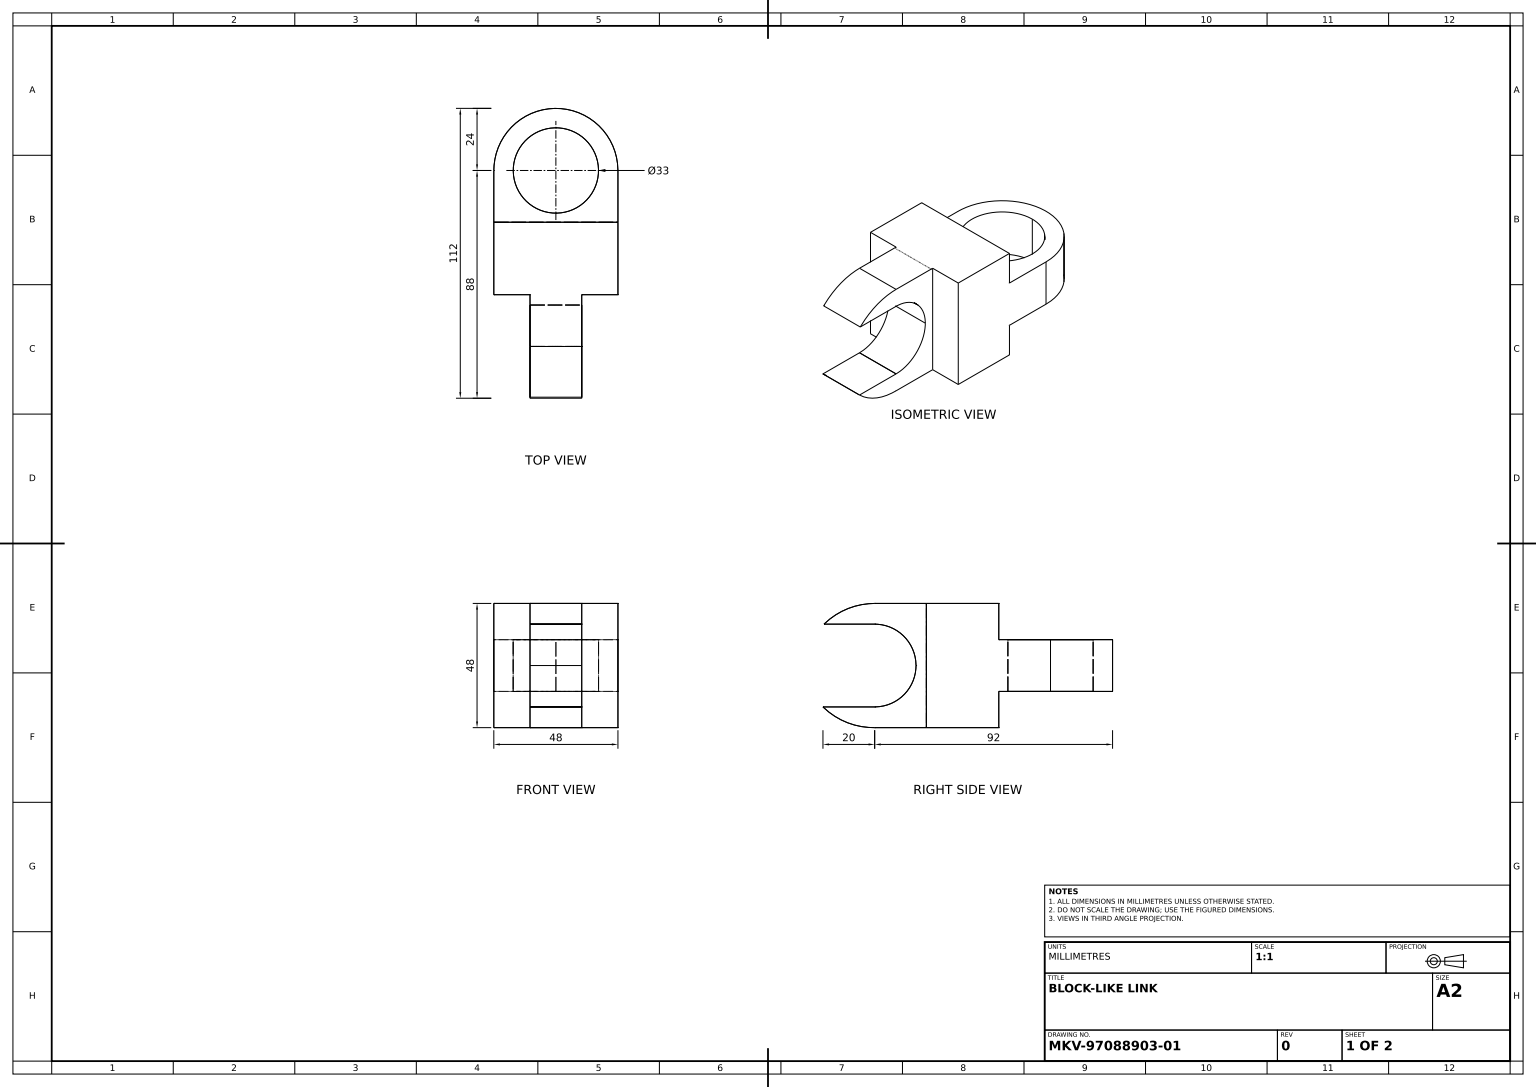
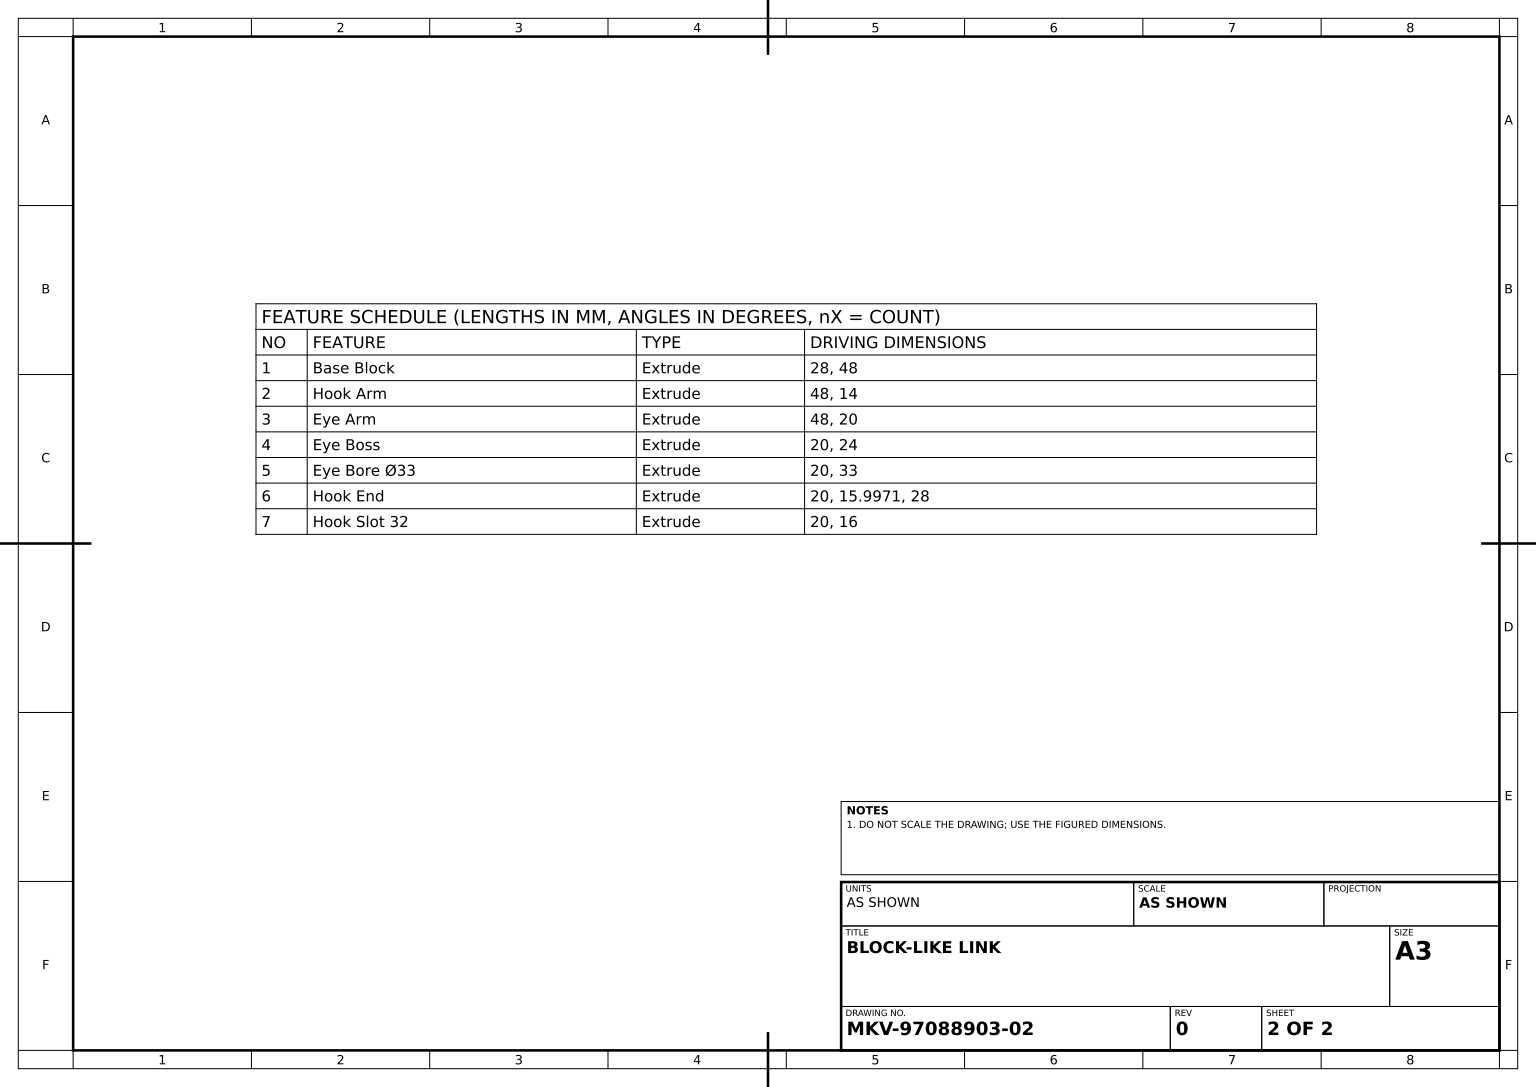
from build123d import *

# Parameters (mm, degrees)
BASE_BLOCK_SKETCH_W = 48
BASE_BLOCK_SKETCH_H = 48
BASE_BLOCK_DEPTH    = 28
HOOK_ARM_DEPTH      = 48
EYE_ARM_DEPTH       = 48
EYE_BOSS_DEPTH      = 20
EYE_BORE_SKETCH_R   = 16.5
EYE_BORE_33_DEPTH   = 20
HOOK_END_DEPTH      = 20
HOOK_SLOT_32_DEPTH  = 20


with BuildPart() as part:
    # Base Block Sketch → Base Block (new body)
    with BuildSketch(Plane.XY):
        with Locations((24, -24)):
            Rectangle(BASE_BLOCK_SKETCH_W, BASE_BLOCK_SKETCH_H)
    extrude(amount=BASE_BLOCK_DEPTH)

    # Hook Arm Sketch → Hook Arm (add)
    with BuildSketch(Plane(origin=(0, 0, 0), x_dir=(1, 0, 0), z_dir=(0, 1, 0))):
        Polygon((34, -28), (24, -28), (14, -28), (14, -48), (34, -48), align=None)
    extrude(amount=-HOOK_ARM_DEPTH)

    # Eye Arm Sketch → Eye Arm (add)
    with BuildSketch(Plane(origin=(48, 0, 0), x_dir=(0, 0, -1), z_dir=(1, 0, 0))):
        Polygon((0, -24), (0, -14), (20, -14), (20, -34), (0, -34), align=None)
    extrude(amount=-EYE_ARM_DEPTH)

    # Eye Boss Sketch → Eye Boss (add)
    with BuildSketch(Plane(origin=(0, -14, 0), x_dir=(1, 0, 0), z_dir=(0, 1, 0))):
        with BuildLine():
            Line((0, 20), (48, 20))
            ThreePointArc((48, 20), (24, 44), (0, 20))
        make_face()
    extrude(amount=-EYE_BOSS_DEPTH)

    # Eye Bore Sketch → Eye Bore Ø33 (cut)
    with BuildSketch(Plane(origin=(0, -14, 0), x_dir=(1, 0, 0), z_dir=(0, 1, 0))):
        with Locations(Location((24, 20, 0), (0, 0, 270))):
            Circle(EYE_BORE_SKETCH_R)
    extrude(amount=-EYE_BORE_33_DEPTH, mode=Mode.SUBTRACT)

    # Hook End Sketch → Hook End (add)
    with BuildSketch(Plane(origin=(34, 0, 0), x_dir=(0, 0, -1), z_dir=(1, 0, 0))):
        with BuildLine():
            Line((-67.598850506, -8.002873735), (-48, -8.002873735))
            Line((-48, -8.002873735), (-48, 0))
            ThreePointArc((-48, 0), (-58.584905871, -2.077813215), (-67.598850506, -8.002873735))
        make_face()
        with BuildLine():
            Line((-48, -48), (-48, -39.997126265))
            Line((-48, -39.997126265), (-68, -39.997126265))
            ThreePointArc((-68, -39.997126265), (-58.800418806, -45.998891596), (-48, -48))
        make_face()
    extrude(amount=-HOOK_END_DEPTH)

    # Hook Slot Sketch → Hook Slot 32 (cut)
    with BuildSketch(Plane(origin=(34, 0, 0), x_dir=(0, 0, -1), z_dir=(1, 0, 0))):
        with BuildLine():
            Line((-48, -8), (-48, -8.002873735))
            Line((-48, -8.002873735), (-48, -39.997126265))
            Line((-48, -39.997126265), (-48, -40))
            ThreePointArc((-48, -40), (-32, -24), (-48, -8))
        make_face()
    extrude(amount=-HOOK_SLOT_32_DEPTH, mode=Mode.SUBTRACT)


solid = part.part
